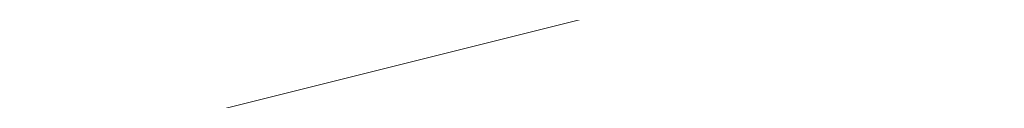
# Model space of a CAD drawing. Units: inches. Extents: x 2091 to 2899, y 967 to 2217.
# Tile 96 of 256: x 2251.2431 to 2251.8124, y 1099.9437 to 1099.9861. Entities that reach past the tile are written whole.
import ezdxf

# ---------------------------------------------------------------- set-up
doc = ezdxf.new("R2010")
doc.units = ezdxf.units.IN
doc.layers.add('A-ANNO-DIMS', color=2, linetype='Continuous', lineweight=18)
doc.layers.add('L-PLNT-TREE', color=94, linetype='Continuous', lineweight=13)
doc.layers.add('A-WALL-PATT', color=141, linetype='Continuous', lineweight=13, true_color=0xadddf7)
doc.styles.get("Standard").update_dxf_attribs({"font": 'arial.ttf'})
doc.dimstyles.new('ISO-25', dxfattribs={"dimtxt": 4, "dimasz": 4, "dimexe": 1.25, "dimexo": 0.625, "dimtad": 1, "dimdec": 0, "dimlunit": 3, "dimtxsty": 'Standard', "dimcen": 2.5, "dimadec": 0, "dimazin": 0, "dimtfac": 1, "dimtdec": 0, "dimtmove": 0, "dimatfit": 3, "dimfxl": 1, "dimarcsym": 0})

# ---------------------------------------------------------------- blocks, each defined once
blk = doc.blocks.new('*U29')
blk.add_line((-402.336, 12.192), (-451.104, 0))
blk = doc.blocks.new('*D71')
at = {"layer": 'A-ANNO-DIMS', "color": 0, "lineweight": -2, "transparency": 16777216}
for p, q in [((2212.1436, 1351.29406), (2212.1436, 969.4643)), ((2452.1436, 1351.29406), (2452.1436, 969.4643)), ((2216.1436, 970.7143), (2448.1436, 970.7143))]:
    blk.add_line(p, q, dxfattribs=at)
at = {"layer": 'A-ANNO-DIMS', "color": 0, "transparency": 16777216}
for points in [[(2216.1436, 971.38097), (2216.1436, 970.04764), (2212.1436, 970.7143)], [(2448.1436, 971.38097), (2448.1436, 970.04764), (2452.1436, 970.7143)]]:
    blk.add_solid(points, dxfattribs=at)
at = {"layer": 'Defpoints', "color": 0, "transparency": 16777216}
for p in [(2212.1436, 1351.91906), (2452.1436, 1351.91906), (2452.1436, 970.7143)]:
    blk.add_point(p, dxfattribs=at)
at = {"layer": 'A-ANNO-DIMS', "color": 0, "transparency": 16777216, "insert": (2332.1436, 973.38159), "char_height": 4, "attachment_point": 5}
blk.add_mtext('20\'-0"', dxfattribs=at)
blk = doc.blocks.new('*D75')
at = {"layer": 'A-ANNO-DIMS', "color": 0, "lineweight": -2, "transparency": 16777216}
for p, q in [((2212.1436, 1274.79406), (2212.1436, 969.4643)), ((2308.1436, 1274.79406), (2308.1436, 969.4643)), ((2216.1436, 970.7143), (2304.1436, 970.7143))]:
    blk.add_line(p, q, dxfattribs=at)
at = {"layer": 'A-ANNO-DIMS', "color": 0, "transparency": 16777216}
for points in [[(2216.1436, 971.38097), (2216.1436, 970.04764), (2212.1436, 970.7143)], [(2304.1436, 971.38097), (2304.1436, 970.04764), (2308.1436, 970.7143)]]:
    blk.add_solid(points, dxfattribs=at)
at = {"layer": 'Defpoints', "color": 0, "transparency": 16777216}
for p in [(2212.1436, 1275.41906), (2308.1436, 1275.41906), (2308.1436, 970.7143)]:
    blk.add_point(p, dxfattribs=at)
at = {"layer": 'A-ANNO-DIMS', "color": 0, "transparency": 16777216, "insert": (2260.1436, 973.38159), "char_height": 4, "attachment_point": 5}
blk.add_mtext('8\'-0"', dxfattribs=at)

msp = doc.modelspace()

# ---------------------------------------------------------------- hatches: boundary and pattern name
at = {"layer": 'A-WALL-PATT'}
h = msp.add_hatch(color=256, dxfattribs=at)
h.dxf.hatch_style = 1
h.paths.add_polyline_path([(2803.1436, 2050.91906), (2203.1436, 2050.91906), (2203.1436, 1090.91906), (2803.1436, 1090.91906)])
h.paths.add_polyline_path([(2635.79885, 1147.54046), (2674.52405, 1147.54046, 0.376086), (2678.52967, 1152.8802), (2678.52967, 1159.55647, 0.333335), (2674.52432, 1163.56185), (2674.52432, 1163.56185), (2674.52432, 1192.93439), (2635.80597, 1192.93439), (2597.08762, 1192.93439), (2597.08762, 1163.56185, 0.333335), (2593.08228, 1159.55647), (2593.08228, 1152.8802, 0.376086), (2597.08789, 1147.54046)], flags=0)
h.paths.add_polyline_path([(2436.01043, 1278.24078, 0.000483), (2435.95264, 1278.21503, -0.001328), (2435.93563, 1278.11169, -0.001711), (2436.11644, 1278.04076, 0.002185)], flags=0)
h.paths.add_polyline_path([(2794.1436, 1143.41906), (2794.1436, 1347.41906), (2543.37017, 1347.41906), (2543.37017, 1351.91906), (2794.1436, 1351.91906), (2794.1436, 1392.71355), (2793.9474, 1392.71355), (2793.9474, 1473.5369), (2794.1436, 1473.5369), (2794.1436, 1531.91906), (2650.1436, 1531.91906), (2650.1436, 1536.41906), (2794.1436, 1536.41906), (2794.1436, 1692.41906), (2609.37561, 1692.41906), (2609.37561, 1644.41906), (2604.87561, 1644.41906), (2604.87561, 1744.91906), (2609.37561, 1744.91906), (2609.37561, 1696.91906), (2794.1436, 1696.91906), (2794.1436, 1780.91906), (2609.6436, 1780.91906), (2493.87561, 1780.91906), (2493.87561, 1785.41906), (2609.6436, 1785.41906), (2794.1436, 1785.41906), (2794.1436, 1847.93882), (2793.95122, 1847.93882), (2793.95122, 1928.76217), (2794.1436, 1928.76217), (2794.1436, 1941.41906), (2614.1436, 1941.41906), (2614.1436, 1821.41906), (2609.6436, 1821.41906), (2609.6436, 1941.41906), (2392.1436, 1941.41906), (2392.1436, 1819.91906), (2387.6436, 1819.91906), (2387.6436, 1941.41906), (2212.1436, 1941.41906), (2212.1436, 1783.91906), (2392.1436, 1783.91906), (2392.1436, 1780.91906), (2212.1436, 1780.91906), (2212.1436, 1629.41906), (2387.6436, 1629.41906), (2387.6436, 1744.91906), (2392.1436, 1744.91906), (2392.1436, 1627.91906), (2317.1436, 1627.91906), (2317.1436, 1551.41906), (2317.1436, 1536.41906), (2459.38359, 1536.41906), (2459.38359, 1602.39648), (2463.88359, 1602.39648), (2463.88359, 1531.91906), (2456.6436, 1531.91906), (2456.6436, 1529.91906), (2452.1436, 1529.91906), (2452.1436, 1531.91906), (2312.6436, 1531.91906), (2312.6436, 1551.41906), (2306.1436, 1551.41906), (2306.1436, 1555.91906), (2308.1436, 1555.91906), (2308.1436, 1551.41906), (2312.6436, 1551.41906), (2312.6436, 1627.91906), (2212.1436, 1627.91906), (2212.1436, 1555.91906), (2270.1436, 1555.91906), (2270.1436, 1551.41906), (2212.1436, 1551.41906), (2212.1436, 1351.91906), (2272.1436, 1351.91906), (2272.1436, 1347.41906), (2212.1436, 1347.41906), (2212.1436, 1275.41906), (2308.1436, 1275.41906), (2308.1436, 1351.91906), (2452.1436, 1351.91906), (2452.1436, 1493.91906), (2456.6436, 1493.91906), (2456.6436, 1347.41906), (2312.6436, 1347.41906), (2312.6436, 1270.91906), (2212.1436, 1270.91906), (2212.1436, 1099.91906), (2281.23752, 1099.91906), (2282.87104, 1110.9138), (2282.00834, 1116.9966), (2278.55774, 1121.4204), (2268.20564, 1128.0562), (2272.08764, 1128.0562), (2273.81294, 1131.927), (2279.42034, 1134.6919), (2285.02784, 1135.2449), (2287.61584, 1137.4568), (2288.04714, 1138.0098), (2289.34114, 1140.7747), (2291.06654, 1139.6687), (2292.36054, 1135.2449), (2295.37984, 1136.9038), (2296.24254, 1135.7979), (2297.10524, 1133.033), (2300.12464, 1138.0098), (2303.14394, 1138.0098), (2304.43794, 1135.7979), (2303.14394, 1133.586), (2306.59464, 1134.6919), (2307.88874, 1133.033), (2310.90804, 1135.2449), (2313.92744, 1134.1389), (2315.62686, 1132.4271), (2308.32004, 1117.5496), (2290.20384, 1109.8079), (2288.90984, 1103.1721), (2289.27231, 1099.91906), (2434.91823, 1099.91906), (2431.59323, 1124.78806), (2429.93023, 1169.55306), (2430.92718, 1240.51969), (2435.65893, 1238.18613), (2437.13523, 1196.55406), (2438.79823, 1143.97306), (2442.67823, 1111.99806), (2446.55823, 1099.91906), (2794.1436, 1099.91906), (2794.1436, 1138.91906), (2548.03245, 1138.91906), (2548.03245, 1143.41906), (2548.03245, 1148.81906), (2546.66846, 1148.03156), (2528.68569, 1179.17862, 0.256256), (2512.03245, 1148.81906), (2512.03245, 1143.41906), (2512.03245, 1138.91906), (2507.53245, 1138.91906), (2507.53245, 1143.41906), (2507.53245, 1148.81906, 0.256256), (2490.8792, 1179.17862), (2472.89644, 1148.03156), (2471.53245, 1148.81906), (2471.53245, 1143.41906), (2467.03245, 1143.41906), (2467.03245, 1269.94579, 0.039061), (2460.90999, 1273.58006), (2467.03245, 1273.58006), (2467.03245, 1286.32536, 0.014511), (2465.21619, 1286.76191), (2467.03245, 1287.05258), (2467.03245, 1323.41906), (2471.53245, 1323.41906), (2471.53245, 1148.81906), (2489.53245, 1179.99597), (2490.89644, 1179.20847), (2490.8792, 1179.17862, -0.256256), (2507.53245, 1148.81906), (2507.53245, 1143.41906), (2512.03245, 1143.41906), (2512.03245, 1148.81906, -0.256256), (2528.68569, 1179.17862), (2528.66846, 1179.20847), (2530.03245, 1179.99597), (2548.03245, 1148.81906), (2548.03245, 1143.41906)], flags=16)
h.paths.add_polyline_path([(2607.76855, 1200.94508), (2607.76855, 1265.03063), (2597.08762, 1281.05201), (2619.78459, 1281.05201), (2627.79528, 1337.12686), (2635.79885, 1337.12686), (2643.81666, 1337.12686), (2651.82736, 1281.05201), (2674.52432, 1281.05201), (2663.8434, 1265.03063), (2663.8434, 1200.94508), (2635.80597, 1200.94508)], flags=0)
edge = h.paths.add_edge_path(flags=0)
edge.add_ellipse((13303.89622, 1272.99872), major_axis=(-10595.31304, 0), ratio=0.84230387009, start_angle=0.628237219, end_angle=0.6465541, ccw=False)
edge.add_ellipse((2711.70045, 1156.85268), major_axis=(2.21977, 0), ratio=0.8423039, start_angle=111.53524, end_angle=180.62824, ccw=False)
edge.add_ellipse((13303.15629, 1272.99872), major_axis=(-10593.02631, 0), ratio=0.84230386954, start_angle=0.528271472, end_angle=0.646554097, ccw=False)
edge.add_line((2710.7646, 1175.3333), (2710.12999, 1175.3333))
edge.add_ellipse((2710.12999, 1176.57978), major_axis=(1.47985, 0), ratio=0.8423039, start_angle=180, end_angle=270, ccw=False)
edge.add_line((2708.65014, 1176.57978), (2708.65014, 1200.78291))
edge.add_ellipse((2710.12999, 1200.78291), major_axis=(1.47985, 0), ratio=0.8423039, start_angle=90, end_angle=180, ccw=False)
edge.add_line((2710.12999, 1202.02939), (2710.46508, 1202.02939))
edge.add_ellipse((13303.15629, 1272.99872), major_axis=(-10593.02631, 0), ratio=0.84230386954, start_angle=-0.090229089, end_angle=0.383866779, ccw=False)
edge.add_ellipse((2710.12999, 1290.92703), major_axis=(-1.47985, 0), ratio=0.8423039, start_angle=0, end_angle=90, ccw=False)
edge.add_line((2708.65014, 1290.92703), (2708.65014, 1315.13017))
edge.add_ellipse((2710.12999, 1315.13017), major_axis=(-1.47985, 0), ratio=0.8423039, start_angle=-90, end_angle=0, ccw=False)
edge.add_line((2710.12999, 1316.37665), (2710.70631, 1316.37665))
edge.add_ellipse((3238.40172, 1296.28957), major_axis=(528.234, 0), ratio=0.84230387, start_angle=176.3495724, end_angle=177.8200497, ccw=False)
edge.add_ellipse((2775.06304, 1071.4507), major_axis=(313.30776, 0), ratio=0.84230387, start_angle=102.1259656, end_angle=103.780529, ccw=False)
edge.add_ellipse((2775.06304, 1078.3057), major_axis=(-305.30289, 0), ratio=0.84230387, start_angle=-79.790461, end_angle=-77.5553727, ccw=False)
edge.add_ellipse((2695.14177, 1541.97538), major_axis=(-250.96022, 0), ratio=0.84230387, start_angle=99.256566, end_angle=102.5549326)
edge.add_line((2741.41033, 1334.21426), (2747.13255, 1337.37848))
edge.add_ellipse((2747.53862, 1336.85748), major_axis=(-0.73992, 0), ratio=0.842304, start_angle=270, end_angle=307.93313, ccw=False)
edge.add_ellipse((2747.53862, 1336.85748), major_axis=(-0.73992, 0), ratio=0.842304, start_angle=232.06687, end_angle=270, ccw=False)
edge.add_line((2747.94469, 1337.37848), (2753.66691, 1334.21426))
edge.add_ellipse((2799.93547, 1541.97538), major_axis=(250.96022, 0), ratio=0.84230387, start_angle=257.4450674, end_angle=260.743434)
edge.add_ellipse((2720.01419, 1078.3057), major_axis=(305.30289, 0), ratio=0.84230387, start_angle=77.5553727, end_angle=79.790461, ccw=False)
edge.add_ellipse((2720.01419, 1071.4507), major_axis=(-313.30776, 0), ratio=0.84230387, start_angle=256.219471, end_angle=257.8740344, ccw=False)
edge.add_ellipse((2256.67551, 1296.28957), major_axis=(-528.234, 0), ratio=0.84230387, start_angle=182.1799503, end_angle=183.6504276, ccw=False)
edge.add_line((2784.37092, 1316.37665), (2784.94725, 1316.37665))
edge.add_ellipse((2784.94725, 1315.13017), major_axis=(1.47985, 0), ratio=0.8423039, start_angle=0, end_angle=90, ccw=False)
edge.add_line((2786.42709, 1315.13017), (2786.42709, 1290.92703))
edge.add_ellipse((2784.94725, 1290.92703), major_axis=(1.47985, 0), ratio=0.8423039, start_angle=270, end_angle=360, ccw=False)
edge.add_ellipse((-7808.07906, 1272.99872), major_axis=(10593.02631, 0), ratio=0.84230386954, start_angle=-0.383866779, end_angle=0.090229089, ccw=False)
edge.add_line((2784.61216, 1202.02939), (2784.94725, 1202.02939))
edge.add_ellipse((2784.94725, 1200.78291), major_axis=(1.47985, 0), ratio=0.8423039, start_angle=0, end_angle=90, ccw=False)
edge.add_line((2786.42709, 1200.78291), (2786.42709, 1176.57978))
edge.add_ellipse((2784.94725, 1176.57978), major_axis=(-1.47985, 0), ratio=0.8423039, start_angle=90, end_angle=180, ccw=False)
edge.add_line((2784.94725, 1175.3333), (2784.31264, 1175.3333))
edge.add_ellipse((-7808.07906, 1272.99872), major_axis=(10593.02631, 0), ratio=0.84230386954, start_angle=-0.618643196, end_angle=-0.528271472, ccw=False)
edge.add_ellipse((2783.37678, 1156.85268), major_axis=(-2.21977, 0), ratio=0.8423039, start_angle=179.37176, end_angle=248.46476, ccw=False)
edge.add_ellipse((-7808.81898, 1272.99872), major_axis=(-10595.31304, 0), ratio=0.84230386576, start_angle=179.353445923, end_angle=179.371762803, ccw=False)
edge.add_ellipse((2780.2973, 1153.50079), major_axis=(-5.24643, 0), ratio=0.8423039, start_angle=90, end_angle=179.35345, ccw=False)
edge.add_line((2780.2973, 1149.08171), (2714.77993, 1149.08171))
edge.add_ellipse((2714.77993, 1153.50079), major_axis=(5.24643, 0), ratio=0.8423039, start_angle=180.64655, end_angle=270, ccw=False)
edge = h.paths.add_edge_path(flags=0)
edge.add_line((2718.18737, 1151.00783), (2718.18737, 1170.47236))
edge.add_ellipse((2721.14706, 1170.47236), major_axis=(-2.95969, 0), ratio=0.8423039, start_angle=-90, end_angle=0, ccw=False)
edge.add_line((2721.14706, 1172.96532), (2773.93017, 1172.96532))
edge.add_ellipse((2773.93017, 1170.47236), major_axis=(-2.95969, 0), ratio=0.8423039, start_angle=180, end_angle=270, ccw=False)
edge.add_line((2776.88987, 1170.47236), (2776.88987, 1151.00783))
edge.add_line((2776.88987, 1151.00783), (2718.18737, 1151.00783))
edge = h.paths.add_edge_path(flags=0)
edge.add_line((2718.18737, 1180.23415), (2718.18737, 1199.05783))
edge.add_ellipse((2747.53862, 1320.39864), major_axis=(147.01792, 0), ratio=0.84230387, start_angle=256.4018653, end_angle=283.5981347)
edge.add_line((2776.88987, 1199.05783), (2776.88987, 1180.23415))
edge.add_ellipse((2747.53862, 1301.57496), major_axis=(147.01792, 0), ratio=0.84230387, start_angle=256.4018653, end_angle=283.5981347, ccw=False)
edge = h.paths.add_edge_path(flags=0)
edge.add_ellipse((13303.15629, 1272.99872), major_axis=(-10591.54646, 0), ratio=0.84230386955, start_angle=0.055594314, end_angle=0.377764194, ccw=False)
edge.add_line((2711.61686, 1262.72171), (2715.66741, 1249.4954))
edge.add_ellipse((6413.89196, 1241.69192), major_axis=(-3698.23616, 0), ratio=0.8423038695, start_angle=-0.12089737, end_angle=0.36407635)
edge.add_line((2715.76104, 1218.19245), (2711.93431, 1203.16736))
edge = h.paths.add_edge_path(flags=0)
edge.add_line((2718.18737, 1251.07457), (2716.00249, 1267.45044))
edge.add_ellipse((2742.15117, 1202.18954), major_axis=(81.77258, 0), ratio=0.84230387, start_angle=94.277421, end_angle=111.8349538, ccw=False)
edge.add_line((2737.00975, 1270.93063), (2758.06748, 1270.93063))
edge.add_ellipse((2752.92606, 1202.18954), major_axis=(81.77258, 0), ratio=0.84230387, start_angle=68.1650462, end_angle=85.722579, ccw=False)
edge.add_line((2779.07475, 1267.45044), (2776.88987, 1251.07457))
edge.add_ellipse((2750.33806, 1187.88536), major_axis=(79.57966, 0), ratio=0.84230387, start_angle=67.2080851, end_angle=85.1299304)
edge.add_line((2756.03466, 1254.74366), (2739.04258, 1254.74366))
edge.add_ellipse((2744.73917, 1187.88536), major_axis=(79.57966, 0), ratio=0.84230387, start_angle=94.8700696, end_angle=112.7919149)
edge = h.paths.add_edge_path(flags=0)
edge.add_line((2783.14293, 1203.16736), (2779.31619, 1218.19245))
edge.add_ellipse((-918.81473, 1241.69192), major_axis=(3698.23616, 0), ratio=0.8423038695, start_angle=-0.36407635, end_angle=0.12089737)
edge.add_line((2779.40983, 1249.4954), (2783.46037, 1262.72171))
edge.add_ellipse((-7808.07906, 1272.99872), major_axis=(-10591.54646, 0), ratio=0.84230386954, start_angle=179.622235806, end_angle=179.944405687, ccw=False)
edge = h.paths.add_edge_path(flags=0)
edge.add_ellipse((2734.20089, 1286.69044), major_axis=(-0.35661, 6.34008), ratio=0.6038336, start_angle=89.002014, end_angle=253.657408, ccw=False)
edge.add_line((2730.369, 1286.54181), (2730.369, 1301.35198))
edge.add_line((2730.369, 1301.35198), (2735.91331, 1305.2148))
edge.add_ellipse((2736.38492, 1304.73456), major_axis=(0.73992, 0), ratio=0.842304, start_angle=90, end_angle=134.48021, ccw=False)
edge.add_line((2736.38492, 1305.3578), (2738.03278, 1305.3578))
edge.add_line((2738.03278, 1305.3578), (2738.03278, 1307.70793))
edge.add_ellipse((2794.20164, 1307.70793), major_axis=(56.16886, 0), ratio=0.84230387, start_angle=150.56143, end_angle=180, ccw=False)
edge.add_ellipse((2700.87559, 1307.70793), major_axis=(-56.16886, 0), ratio=0.84230387, start_angle=180, end_angle=209.43857, ccw=False)
edge.add_line((2757.04445, 1307.70793), (2757.04445, 1305.3578))
edge.add_line((2757.04445, 1305.3578), (2758.69232, 1305.3578))
edge.add_ellipse((2758.69232, 1304.73456), major_axis=(-0.73992, 0), ratio=0.842304, start_angle=225.51979, end_angle=270, ccw=False)
edge.add_line((2759.16392, 1305.2148), (2764.70823, 1301.35198))
edge.add_line((2764.70823, 1301.35198), (2764.70823, 1286.54181))
edge.add_ellipse((2760.87634, 1286.69044), major_axis=(0.35661, 6.34008), ratio=0.6038336, start_angle=106.342592, end_angle=270.997986, ccw=False)
edge.add_line((2757.04445, 1285.79709), (2757.04445, 1307.70793))
edge.add_ellipse((2700.87559, 1307.70793), major_axis=(-56.16886, 0), ratio=0.84230387, start_angle=180, end_angle=209.43857)
edge.add_ellipse((2794.20164, 1307.70793), major_axis=(56.16886, 0), ratio=0.84230387, start_angle=150.56143, end_angle=180)
edge.add_line((2738.03278, 1307.70793), (2738.03278, 1285.79709))
h.paths.add_polyline_path([(2417.81227, 1104.4497), (2413.49227, 1102.5297), (2410.61227, 1103.9697), (2409.17227, 1106.3697), (2407.25227, 1107.3297), (2406.29227, 1109.7297), (2405.33227, 1114.0497), (2405.33227, 1117.8897), (2406.29227, 1120.1297), (2407.25227, 1119.8097), (2408.84832, 1118.32766), (2410.17395, 1119.42417), (2410.21127, 1120.4057), (2411.04073, 1121.41905), (2410.69927, 1119.8587), (2410.17395, 1119.42417), (2410.08845, 1117.17611), (2411.13284, 1116.20632), (2413.97227, 1119.3297), (2416.85227, 1120.7697), (2416.86972, 1120.79878), (2417.03507, 1119.40512), (2417.89621, 1118.14338), (2418.29227, 1118.3697), (2419.54445, 1120.03927), (2419.36092, 1118.38749), (2419.03211, 1119.35615), (2418.39894, 1118.51193), (2419.25227, 1114.5297), (2418.79409, 1107.19879)], flags=0)
h.paths.add_polyline_path([(2508.87017, 1347.41906), (2508.37017, 1347.41906), (2508.37017, 1351.91906), (2508.87017, 1351.91906)], flags=0)
h.paths.add_polyline_path([(2473.37017, 1347.41906), (2472.37017, 1347.41906), (2467.87017, 1347.41906), (2467.87017, 1455.41906), (2472.37017, 1455.41906), (2472.37017, 1352.41906), (2473.37017, 1352.41906)], flags=0)
h.paths.add_polyline_path([(2352.10624, 1217.4462), (2349.22624, 1218.8862), (2347.78624, 1221.2862), (2345.86624, 1222.2462), (2344.90624, 1224.6462), (2343.94624, 1228.9662), (2343.94624, 1232.8062), (2344.90624, 1235.0462), (2345.86624, 1234.7262), (2347.46229, 1233.24415), (2348.78792, 1234.34066), (2348.82524, 1235.3222), (2349.6547, 1236.33555), (2349.31324, 1234.7752), (2348.78792, 1234.34066), (2348.70242, 1232.0926), (2349.74681, 1231.12282), (2352.58624, 1234.2462), (2355.46624, 1235.6862), (2355.48369, 1235.71528), (2355.64904, 1234.32161), (2356.51018, 1233.05988), (2356.90624, 1233.2862), (2358.15842, 1234.95576), (2357.97489, 1233.30398), (2357.64608, 1234.27264), (2357.01291, 1233.42842), (2357.86624, 1229.4462), (2357.40806, 1222.11529), (2356.42624, 1219.3662)], flags=0)
h.paths.add_polyline_path([(2348.2968, 1112.22442), (2347.0138, 1112.31042), (2345.5298, 1114.12742), (2345.7318, 1115.85842), (2346.8118, 1116.98242), (2346.8118, 1114.64642), (2345.8668, 1114.21442), (2346.8798, 1114.30042)], flags=0)
h.paths.add_polyline_path([(2347.0138, 1110.92642), (2346.2718, 1110.49342), (2346.6098, 1111.18642)], flags=0)
h.paths.add_polyline_path([(2345.8668, 1118.19442), (2345.5298, 1117.32942), (2343.7078, 1118.02142), (2344.3828, 1118.62642)], flags=0)
h.paths.add_polyline_path([(2346.6768, 1109.28242), (2346.0698, 1108.07142), (2345.8668, 1110.06142)], flags=0)
h.paths.add_polyline_path([(2345.0568, 1119.75142), (2343.6398, 1119.75142), (2343.9778, 1121.13542)], flags=0)
h.paths.add_polyline_path([(2345.2598, 1116.55042), (2345.1248, 1115.85842), (2344.9218, 1115.68542), (2344.7198, 1116.37742)], flags=0)
h.paths.add_polyline_path([(2345.6648, 1112.31042), (2345.4618, 1111.53242), (2344.0448, 1111.96442), (2344.6518, 1112.57042)], flags=0)
h.paths.add_polyline_path([(2345.1918, 1113.34942), (2344.4498, 1113.86842), (2344.7198, 1114.38742)], flags=0)
h.paths.add_polyline_path([(2344.6518, 1116.80942), (2344.1798, 1115.68542), (2344.6518, 1115.33942), (2343.9098, 1114.90642), (2343.0328, 1115.94442), (2343.6398, 1116.46342)], flags=0)
h.paths.add_polyline_path([(2345.8668, 1106.68642), (2344.9898, 1105.56242), (2344.5168, 1106.60042)], flags=0)
h.paths.add_polyline_path([(2344.8548, 1110.06142), (2344.5168, 1109.28242), (2344.1128, 1109.71542)], flags=0)
h.paths.add_polyline_path([(2344.0448, 1113.52242), (2343.4378, 1113.08942), (2342.7628, 1113.95442)], flags=0)
h.paths.add_polyline_path([(2344.3148, 1111.01242), (2342.9648, 1110.32042), (2342.9648, 1111.09942)], flags=0)
h.paths.add_polyline_path([(2345.1248, 1104.69742), (2344.5848, 1103.74542), (2344.4498, 1104.26442)], flags=0)
h.paths.add_polyline_path([(2342.8298, 1121.22242), (2341.7498, 1120.53042), (2340.5358, 1121.04942), (2340.1308, 1121.82842), (2340.6708, 1122.95242), (2341.1428, 1121.82842), (2341.6148, 1122.00142)], flags=0)
h.paths.add_polyline_path([(2342.9648, 1119.75142), (2343.0328, 1118.45342), (2342.0878, 1118.02142), (2342.0198, 1119.49142)], flags=0)
h.paths.add_polyline_path([(2342.6948, 1116.89642), (2341.9528, 1116.63642), (2342.0198, 1117.32942)], flags=0)
h.paths.add_polyline_path([(2343.0328, 1112.22442), (2342.0198, 1111.79142), (2341.5478, 1112.22442), (2342.3578, 1113.34942)], flags=0)
h.paths.add_polyline_path([(2343.7748, 1104.43742), (2342.6278, 1102.88042), (2342.6948, 1104.61042), (2343.4378, 1105.12942)], flags=0)
h.paths.add_polyline_path([(2342.0198, 1115.07942), (2340.8058, 1115.51242), (2340.9408, 1116.37742)], flags=0)
h.paths.add_polyline_path([(2341.4808, 1120.09742), (2341.4808, 1119.40542), (2341.0758, 1119.57842), (2341.1428, 1120.09742)], flags=0)
h.paths.add_polyline_path([(2341.8178, 1114.47342), (2340.9408, 1113.08942), (2340.8058, 1114.56042)], flags=0)
h.paths.add_polyline_path([(2341.1428, 1118.54042), (2340.9408, 1116.98242), (2339.0508, 1117.67542), (2339.0508, 1118.62642)], flags=0)
h.paths.add_polyline_path([(2342.6948, 1101.66842), (2341.9528, 1101.84142), (2342.5598, 1102.36142)], flags=0)
h.paths.add_polyline_path([(2340.3328, 1119.66542), (2338.4438, 1119.57842), (2337.9038, 1120.35742), (2339.6578, 1120.61642)], flags=0)
h.paths.add_polyline_path([(2340.3328, 1115.33942), (2340.0628, 1113.69542), (2339.3878, 1115.33942)], flags=0)
h.paths.add_polyline_path([(2341.8178, 1103.83142), (2341.5478, 1102.88042), (2341.1428, 1103.65842)], flags=0)
h.paths.add_polyline_path([(2339.0508, 1122.86642), (2337.2958, 1121.82842), (2337.0938, 1123.12542), (2337.7688, 1123.81842)], flags=0)
h.paths.add_polyline_path([(2339.1178, 1121.74142), (2338.8478, 1121.22242), (2338.1738, 1121.04942), (2338.3758, 1121.56842)], flags=0)
h.paths.add_polyline_path([(2339.1858, 1119.31942), (2338.6458, 1118.71342), (2338.2408, 1118.10742), (2338.2408, 1118.88642)], flags=0)
h.paths.add_polyline_path([(2341.1428, 1101.92842), (2340.6028, 1101.23642), (2340.0628, 1101.84142), (2340.6028, 1102.36142)], flags=0)
h.paths.add_polyline_path([(2337.6338, 1117.76142), (2336.6208, 1118.28042), (2337.2958, 1118.97242)], flags=0)
h.paths.add_polyline_path([(2336.8238, 1119.57842), (2334.7988, 1118.97242), (2335.2038, 1120.35742), (2336.5538, 1120.87642)], flags=0)
h.paths.add_polyline_path([(2339.1178, 1100.45742), (2337.3638, 1100.54342), (2336.7558, 1101.23642)], flags=0)
h.paths.add_polyline_path([(2336.3508, 1122.43342), (2336.0138, 1121.91442), (2334.9338, 1122.43342), (2334.5288, 1123.47142), (2335.7438, 1122.77942)], flags=0)
h.paths.add_polyline_path([(2334.7318, 1120.87642), (2334.2588, 1120.35742), (2334.0568, 1120.78942), (2334.5968, 1121.30842)], flags=0)
h.paths.add_polyline_path([(2334.4618, 1122.17442), (2332.5718, 1121.30842), (2331.3568, 1122.17442), (2332.0998, 1122.86642)], flags=0)
h.paths.add_polyline_path([(2334.2588, 1118.54042), (2333.3818, 1118.45342), (2333.6518, 1119.31942)], flags=0)
h.paths.add_polyline_path([(2335.5418, 1102.27442), (2334.1918, 1102.62042), (2335.2718, 1103.31242)], flags=0)
h.paths.add_polyline_path([(2332.7068, 1119.66542), (2331.6948, 1120.44342), (2332.5048, 1120.78942)], flags=0)
h.paths.add_polyline_path([(2334.7318, 1101.14942), (2333.5168, 1101.58242), (2333.9888, 1101.75542)], flags=0)
h.paths.add_polyline_path([(2332.6398, 1116.63642), (2331.0868, 1116.29042), (2331.9648, 1118.19442)], flags=0)
h.paths.add_polyline_path([(2330.7498, 1121.56842), (2330.2768, 1120.27042), (2328.5228, 1119.31942), (2328.9948, 1121.04942)], flags=0)
h.paths.add_polyline_path([(2330.7498, 1118.62642), (2330.0078, 1117.50242), (2329.8728, 1118.02142)], flags=0)
h.paths.add_polyline_path([(2332.0998, 1102.36142), (2330.5468, 1102.01442), (2331.6948, 1102.96642)], flags=0)
h.paths.add_polyline_path([(2329.5348, 1113.60842), (2329.0628, 1112.31042), (2328.5898, 1113.34942)], flags=0)
h.paths.add_polyline_path([(2328.3878, 1117.84842), (2327.5098, 1116.55042), (2327.1728, 1117.76142)], flags=0)
h.paths.add_polyline_path([(2329.7378, 1106.51342), (2329.5348, 1105.30242), (2328.2528, 1106.08142)], flags=0)
h.paths.add_polyline_path([(2328.6578, 1114.38742), (2328.0498, 1114.12742), (2328.3198, 1114.90642)], flags=0)
h.paths.add_polyline_path([(2328.3198, 1112.22442), (2327.1058, 1112.13742), (2326.7008, 1112.65642)], flags=0)
h.paths.add_polyline_path([(2326.9028, 1115.25242), (2326.7008, 1114.12742), (2325.2158, 1113.60842), (2326.0928, 1115.33942)], flags=0)
h.paths.add_polyline_path([(2326.6328, 1108.33042), (2326.0928, 1107.37942), (2325.8908, 1108.50342), (2326.4978, 1109.10942)], flags=0)
h.paths.add_polyline_path([(2615.1436, 1531.91906), (2609.6436, 1531.91906), (2609.6436, 1620.41906), (2614.1436, 1620.41906), (2614.1436, 1536.41906), (2615.1436, 1536.41906)], flags=0)
h.paths.add_polyline_path([(2545.1436, 1563.41906), (2464.1436, 1563.41906), (2464.1436, 1632.41906), (2509.1436, 1632.41906), (2509.1436, 1627.91906), (2509.1436, 1603.91906), (2468.6436, 1603.91906), (2468.6436, 1567.91906), (2540.6436, 1567.91906), (2540.6436, 1591.91906), (2545.1436, 1591.91906)], flags=0)
h.paths.add_polyline_path([(2388.96905, 1549.98573), (2357.43418, 1549.98573), (2357.43418, 1623.36078), (2399.36278, 1623.36078), (2435.68947, 1623.36078), (2435.59255, 1602.55927), (2435.59255, 1602.39648), (2388.96905, 1602.39648)], flags=0)
h.paths.add_polyline_path([(2388.88063, 1555.80915), (2374.90443, 1555.80915), (2374.90443, 1600.57156), (2374.90443, 1615.45765), (2406.35088, 1615.45765), (2406.35088, 1618.93943), (2412.17429, 1615.45765), (2406.35088, 1611.97586), (2406.35088, 1615.45765), (2388.88063, 1615.45765)], flags=0)
h.paths.add_polyline_path([(2568.87561, 1644.41906), (2453.37561, 1644.41906), (2453.37561, 1785.41906), (2457.87561, 1785.41906), (2457.87561, 1648.91906), (2568.87561, 1648.91906)], flags=0)
h.paths.add_polyline_path([(2212.1436, 1945.91906), (2212.1436, 2041.91906), (2794.1436, 2041.91906), (2794.1436, 1945.91906)], flags=16)
h.paths.add_polyline_path([(2271.08273, 1964.31724), (2776.85297, 1964.31724), (2776.85297, 2037.16962), (2271.08273, 2037.16962)], flags=8)
h.paths.add_polyline_path([(2380.64929, 1536.82414), (2461.04081, 1536.82414), (2461.04081, 1554.65259), (2380.64929, 1554.65259)], flags=8)
h.paths.add_polyline_path([(2240.75571, 1609.72545), (2309.18583, 1609.72545), (2309.18583, 1617.6982), (2240.75571, 1617.6982)], flags=8)
h.paths.add_polyline_path([(2212.67726, 1313.5041), (2282.59152, 1313.5041), (2282.59152, 1322.74524), (2212.67726, 1322.74524)], flags=8)
h.paths.add_polyline_path([(2457.11198, 1114.77857), (2558.48158, 1114.77857), (2558.48158, 1142.21968), (2457.11198, 1142.21968)], flags=8)
h.paths.add_polyline_path([(2473.44234, 1273.01007), (2604.64123, 1273.01007), (2604.64123, 1318.34693), (2473.44234, 1318.34693)], flags=8)
h.paths.add_polyline_path([(2638.8763, 1626.97743), (2684.25037, 1627.97674), (2684.03848, 1637.59749), (2638.66442, 1636.59819)], flags=8)
h.paths.add_polyline_path([(2537.59055, 1453.79345), (2628.38955, 1453.79345), (2628.38955, 1475.34481), (2537.59055, 1475.34481)], flags=8)
h.paths.add_polyline_path([(2504.13764, 1714.6324), (2554.64719, 1714.6324), (2554.64719, 1730.23771), (2504.13764, 1730.23771)], flags=8)
h.paths.add_polyline_path([(2487.50118, 1575.65187), (2535.09712, 1575.65187), (2535.09712, 1598.37765), (2487.50118, 1598.37765)], flags=8)
h.paths.add_polyline_path([(2709.0994, 1735.71028), (2740.0166, 1735.71028), (2740.0166, 1749.93764), (2709.0994, 1749.93764)], flags=8)
h.paths.add_polyline_path([(2442.43842, 1792.17166), (2564.72884, 1792.17166), (2564.72884, 1842.00016), (2442.43842, 1842.00016)], flags=8)
h.paths.add_polyline_path([(2655.8158, 1809.64408), (2789.52014, 1806.6938), (2790.08498, 1832.29164), (2656.38064, 1835.24192)], flags=8)
h.paths.add_polyline_path([(2234.8427, 1797.72014), (2368.59285, 1794.76885), (2369.16072, 1820.50413), (2235.41056, 1823.45542)], flags=8)
h.paths.add_polyline_path([(2245.13847, 1644.00633), (2398.42773, 1640.6239), (2398.99484, 1666.32482), (2245.70557, 1669.70725)], flags=8)
h.paths.add_polyline_path([(2306.14285, 1431.16852), (2413.76831, 1428.79369), (2414.33315, 1454.39153), (2306.70768, 1456.76636)], flags=8)
h.paths.add_polyline_path([(2306.83458, 1458.23314), (2393.38048, 1456.32345), (2393.93281, 1481.35436), (2307.38691, 1483.26405)], flags=8)

# ---------------------------------------------------------------- block references
at = {"layer": 'L-PLNT-TREE', "xscale": 0.0393700787401575, "yscale": 0.0393700787401575, "zscale": 0.0393700787401575}
msp.add_blockref('*U29', (2269.04101, 1099.91906), dxfattribs=at)

# ---------------------------------------------------------------- dimensions: what is measured, and where the dimension line sits
at = {"layer": 'A-ANNO-DIMS'}
for base, p1, p2, picture, middle in [((2452.1436, 970.7143), (2212.1436, 1351.91906), (2452.1436, 1351.91906), '*D71', (2332.1436, 973.38159)), ((2308.1436, 970.7143), (2212.1436, 1275.41906), (2308.1436, 1275.41906), '*D75', (2260.1436, 973.38159))]:
    dim = msp.add_linear_dim(base=base, p1=p1, p2=p2, dimstyle='ISO-25', override={"dimdec": 1, "dimlfac": 1, "dimrnd": 0, "dimzin": 1, "dimdsep": 46, "dimlunit": 4, "dimfrac": 2}, dxfattribs=at)
    dim.commit()
    dim.dimension.update_dxf_attribs({"geometry": picture, "text_midpoint": middle})

doc.saveas('drawing.dxf')
